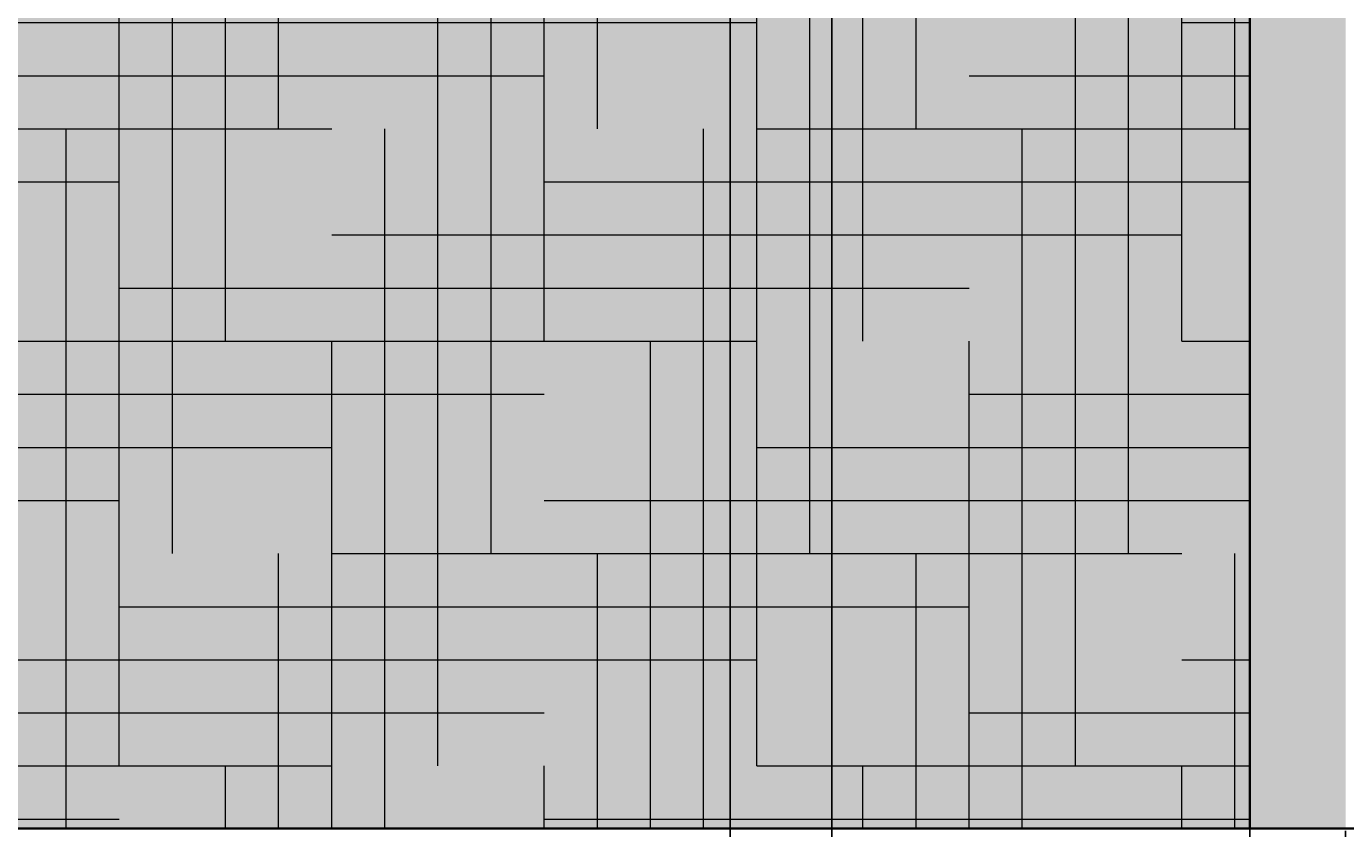
# Model space of a CAD drawing. Units: feet. Extents: x 2695 to 2912, y 795 to 1139.
# Tile 4 of 83: x 2734 to 2774, y 811 to 835. Entities that reach past the tile are written whole.
import ezdxf

# ---------------------------------------------------------------- set-up
doc = ezdxf.new("R2010")
doc.units = ezdxf.units.FT
for name, color, linetype, lineweight in [('A-ANNO-DIMS', 2, 'Continuous', 18), ('A-ELEV', 7, 'Continuous', 35), ('A-ELEV-PATT', 252, 'Continuous', 13)]:
    doc.layers.add(name, color=color, linetype=linetype, lineweight=lineweight)
doc.styles.get("Standard").update_dxf_attribs({"font": 'arial.ttf'})
doc.dimstyles.get("Standard").update_dxf_attribs({"dimtxt": 0.18, "dimasz": 0.18, "dimexe": 0.18, "dimexo": 0.0625, "dimgap": 0.09, "dimtad": 0, "dimtih": 1, "dimtoh": 1, "dimdec": 1, "dimzin": 0, "dimdsep": 46, "dimlunit": 3, "dimtxsty": 'Standard', "dimcen": 0.09, "dimadec": 0, "dimazin": 0, "dimtfac": 1, "dimtdec": 1, "dimtofl": 0, "dimtmove": 0, "dimatfit": 3, "dimfxl": 1, "dimtolj": 1, "dimtzin": 0, "dimarcsym": 0})

# ---------------------------------------------------------------- blocks, each defined once
blk = doc.blocks.new('*D3')
at = {"layer": 'A-ANNO-DIMS', "color": 0, "lineweight": -2, "transparency": 16777216}
for p, q in [((2724.189, 874.795), (2724.189, 794.976)), ((2758.151, 874.795), (2758.151, 794.976)), ((2724.369, 795.156), (2740.777, 795.156)), ((2757.971, 795.156), (2741.564, 795.156))]:
    blk.add_line(p, q, dxfattribs=at)
at = {"layer": 'A-ANNO-DIMS', "color": 0, "transparency": 16777216}
for points in [[(2724.369, 795.186), (2724.369, 795.126), (2724.189, 795.156)], [(2757.971, 795.186), (2757.971, 795.126), (2758.151, 795.156)]]:
    blk.add_solid(points, dxfattribs=at)
at = {"layer": 'Defpoints', "color": 0, "transparency": 16777216}
for p in [(2724.189, 874.857), (2758.151, 874.857), (2758.151, 795.156)]:
    blk.add_point(p, dxfattribs=at)
at = {"layer": 'A-ANNO-DIMS', "color": 0, "transparency": 16777216, "insert": (2741.17, 795.156), "char_height": 0.18, "attachment_point": 5}
blk.add_mtext('\\A1;33.96', dxfattribs=at)
blk = doc.blocks.new('*D4')
at = {"layer": 'A-ANNO-DIMS', "color": 0, "lineweight": -2, "transparency": 16777216}
for p, q in [((2758.151, 874.795), (2758.151, 794.976)), ((2773.503, 810.868), (2773.503, 794.976)), ((2758.331, 795.156), (2765.441, 795.156)), ((2773.323, 795.156), (2766.213, 795.156))]:
    blk.add_line(p, q, dxfattribs=at)
at = {"layer": 'A-ANNO-DIMS', "color": 0, "transparency": 16777216}
for points in [[(2758.331, 795.186), (2758.331, 795.126), (2758.151, 795.156)], [(2773.323, 795.186), (2773.323, 795.126), (2773.503, 795.156)]]:
    blk.add_solid(points, dxfattribs=at)
at = {"layer": 'Defpoints', "color": 0, "transparency": 16777216}
for p in [(2758.151, 874.857), (2773.503, 810.931), (2773.503, 795.156)]:
    blk.add_point(p, dxfattribs=at)
at = {"layer": 'A-ANNO-DIMS', "color": 0, "transparency": 16777216, "insert": (2765.827, 795.156), "char_height": 0.18, "attachment_point": 5}
blk.add_mtext('\\A1;15.35', dxfattribs=at)
blk = doc.blocks.new('*D13')
at = {"layer": 'A-ANNO-DIMS', "color": 0, "lineweight": -2, "transparency": 16777216}
for p, q in [((2758.214, 874.857), (2911.424, 874.857)), ((2911.244, 874.677), (2911.244, 843.076)), ((2911.244, 811.111), (2911.244, 842.712)), ((2890.699, 810.931), (2911.424, 810.931))]:
    blk.add_line(p, q, dxfattribs=at)
at = {"layer": 'A-ANNO-DIMS', "color": 0, "transparency": 16777216}
for points in [[(2911.214, 874.677), (2911.274, 874.677), (2911.244, 874.857)], [(2911.214, 811.111), (2911.274, 811.111), (2911.244, 810.931)]]:
    blk.add_solid(points, dxfattribs=at)
at = {"layer": 'Defpoints', "color": 0, "transparency": 16777216}
for p in [(2758.151, 874.857), (2911.244, 874.857), (2890.636, 810.931)]:
    blk.add_point(p, dxfattribs=at)
at = {"layer": 'A-ANNO-DIMS', "color": 0, "transparency": 16777216, "insert": (2911.244, 842.894), "char_height": 0.18, "attachment_point": 5}
blk.add_mtext('\\A1;63.93', dxfattribs=at)
blk = doc.blocks.new('*D24')
at = {"layer": 'A-ANNO-DIMS', "color": 0, "lineweight": -2, "transparency": 16777216}
for p, q in [((2730.708, 936.868), (2730.708, 794.976)), ((2755.112, 936.868), (2755.112, 794.976)), ((2730.888, 795.156), (2742.446, 795.156)), ((2754.932, 795.156), (2743.375, 795.156))]:
    blk.add_line(p, q, dxfattribs=at)
at = {"layer": 'A-ANNO-DIMS', "color": 0, "transparency": 16777216}
for points in [[(2730.888, 795.186), (2730.888, 795.126), (2730.708, 795.156)], [(2754.932, 795.186), (2754.932, 795.126), (2755.112, 795.156)]]:
    blk.add_solid(points, dxfattribs=at)
at = {"layer": 'Defpoints', "color": 0, "transparency": 16777216}
for p in [(2730.708, 936.931), (2755.112, 936.931), (2755.112, 795.156)]:
    blk.add_point(p, dxfattribs=at)
at = {"layer": 'A-ANNO-DIMS', "color": 0, "transparency": 16777216, "insert": (2742.91, 795.156), "char_height": 0.18, "attachment_point": 5}
blk.add_mtext('\\A1;24.404', dxfattribs=at)
blk = doc.blocks.new('*D25')
at = {"layer": 'A-ANNO-DIMS', "color": 0, "lineweight": -2, "transparency": 16777216}
for p, q in [((2755.112, 936.868), (2755.112, 794.976)), ((2770.636, 936.868), (2770.636, 794.976)), ((2755.292, 795.156), (2762.419, 795.156)), ((2770.456, 795.156), (2763.329, 795.156))]:
    blk.add_line(p, q, dxfattribs=at)
at = {"layer": 'A-ANNO-DIMS', "color": 0, "transparency": 16777216}
for points in [[(2755.292, 795.186), (2755.292, 795.126), (2755.112, 795.156)], [(2770.456, 795.186), (2770.456, 795.126), (2770.636, 795.156)]]:
    blk.add_solid(points, dxfattribs=at)
at = {"layer": 'Defpoints', "color": 0, "transparency": 16777216}
for p in [(2755.112, 936.931), (2770.636, 936.931), (2770.636, 795.156)]:
    blk.add_point(p, dxfattribs=at)
at = {"layer": 'A-ANNO-DIMS', "color": 0, "transparency": 16777216, "insert": (2762.874, 795.156), "char_height": 0.18, "attachment_point": 5}
blk.add_mtext('\\A1;15.524', dxfattribs=at)

msp = doc.modelspace()

# ---------------------------------------------------------------- hatches: boundary and pattern name
at = {"layer": 'A-ELEV-PATT'}
h = msp.add_hatch(color=256, dxfattribs=at)
h.set_gradient(color1=(147, 149, 152), color2=(147, 149, 152), tint=1)
h.paths.add_polyline_path([(2770.6361, 1118.4096), (2710.6361, 1118.4096), (2710.6361, 1062.9306), (2770.6361, 1062.9306)])
h.paths.add_polyline_path([(2890.6361, 1103.3378), (2770.6361, 1103.3378), (2770.6361, 1062.9306), (2890.6361, 1062.9306)])
h.paths.add_polyline_path([(2730.7081, 1048.1052), (2755.1125, 1048.1052), (2755.1125, 936.9306), (2770.6361, 936.9306), (2770.6361, 1050.3105), (2715.8852, 1050.3105), (2715.8852, 936.9306), (2730.7081, 936.9306)])
h.paths.add_polyline_path([(2890.6361, 1050.3105), (2770.6361, 1050.3105), (2770.6361, 971.9673), (2778.0341, 971.9673), (2778.0341, 1020.8235), (2843.575, 1020.8235), (2843.575, 971.9673), (2890.6361, 971.9673)])
h.paths.add_polyline_path([(2888.1882, 970.7156), (2843.575, 970.7156), (2843.575, 964.8267), (2888.1882, 964.8267)])
h.paths.add_polyline_path([(2888.1882, 964.1328), (2843.575, 964.1328), (2843.575, 956.614), (2888.1882, 956.614)])
h.paths.add_polyline_path([(2888.1882, 955.9202), (2843.575, 955.9202), (2843.575, 949.2892), (2888.1882, 949.2892)])
h.paths.add_polyline_path([(2888.1882, 948.5954), (2843.575, 948.5954), (2843.575, 941.3507), (2888.1882, 941.3507)])
h.paths.add_polyline_path([(2888.1882, 940.6569), (2843.575, 940.6569), (2843.575, 936.9306), (2888.1882, 936.9306)])
h.paths.add_polyline_path([(2890.6361, 970.7156), (2888.9368, 970.7156), (2888.9368, 964.8267), (2890.6361, 964.8267)])
h.paths.add_polyline_path([(2890.6361, 964.1328), (2888.9368, 964.1328), (2888.9368, 956.614), (2890.6361, 956.614)])
h.paths.add_polyline_path([(2890.6361, 955.9202), (2888.9368, 955.9202), (2888.9368, 949.2892), (2890.6361, 949.2892)])
h.paths.add_polyline_path([(2890.6361, 940.6569), (2888.9368, 940.6569), (2888.9368, 936.9306), (2890.6361, 936.9306)])
h.paths.add_polyline_path([(2890.6361, 948.5954), (2888.9368, 948.5954), (2888.9368, 941.3507), (2890.6361, 941.3507)])
h.paths.add_polyline_path([(2772.5216, 970.7156), (2770.6361, 970.7156), (2770.6361, 964.8267), (2772.5216, 964.8267)])
h.paths.add_polyline_path([(2772.5216, 964.1328), (2770.6361, 964.1328), (2770.6361, 956.614), (2772.5216, 956.614)])
h.paths.add_polyline_path([(2772.5216, 955.9202), (2770.6361, 955.9202), (2770.6361, 949.2892), (2772.5216, 949.2892)])
h.paths.add_polyline_path([(2772.5216, 948.5954), (2770.6361, 948.5954), (2770.6361, 941.3507), (2772.5216, 941.3507)])
h.paths.add_polyline_path([(2772.5216, 940.6569), (2770.6361, 940.6569), (2770.6361, 936.9306), (2772.5216, 936.9306)])
h.paths.add_polyline_path([(2778.0341, 940.6569), (2773.2702, 940.6569), (2773.2702, 936.9306), (2778.0341, 936.9306)])
h.paths.add_polyline_path([(2778.0341, 970.7156), (2773.2702, 970.7156), (2773.2702, 964.8267), (2778.0341, 964.8267)])
h.paths.add_polyline_path([(2778.0341, 964.1328), (2773.2702, 964.1328), (2773.2702, 956.614), (2778.0341, 956.614)])
h.paths.add_polyline_path([(2778.0341, 955.9202), (2773.2702, 955.9202), (2773.2702, 949.2892), (2778.0341, 949.2892)])
h.paths.add_polyline_path([(2778.0341, 948.5954), (2773.2702, 948.5954), (2773.2702, 941.3507), (2778.0341, 941.3507)])
h.paths.add_polyline_path([(2810.0407, 940.6569), (2780.0341, 940.6569), (2780.0341, 936.9306), (2810.0407, 936.9306)])
h.paths.add_polyline_path([(2890.6361, 924.3105), (2770.6361, 924.3105), (2770.6361, 810.9306), (2773.5029, 810.9306), (2773.5029, 905.5143), (2805.9398, 905.5143), (2838.3767, 905.5143), (2838.3767, 810.9306), (2890.6361, 810.9306)])
h = msp.add_hatch(color=256, dxfattribs=at)
h.set_gradient(color1=(255, 255, 255))
h.paths.add_polyline_path([(2770.6361, 924.3105), (2716.5358, 924.3105), (2716.5358, 810.9306), (2770.6361, 810.9306)])
h.paths.add_polyline_path([(2758.1515, 902.577), (2758.1515, 874.8571), (2724.1893, 874.8571), (2724.1893, 902.577)], flags=16)
h.paths.add_polyline_path([(2756.1515, 900.577), (2756.1515, 876.8571), (2726.1893, 876.8571), (2726.1893, 900.577)], flags=0)
h.paths.add_polyline_path([(2740.7302, 900.577), (2741.6105, 900.577), (2741.6105, 876.8571), (2740.7302, 876.8571)], flags=0)
h = msp.add_hatch(dxfattribs=at)
h.set_pattern_fill('HOUND', color=256, style=0)
h.paths.add_polyline_path([(2770.6361, 924.3105), (2716.5358, 924.3105), (2716.5358, 810.9306), (2770.6361, 810.9306)])
h.paths.add_polyline_path([(2724.1893, 874.8571), (2724.1893, 902.577), (2758.1515, 902.577), (2758.1515, 874.8571)], flags=16)
h.paths.add_polyline_path([(2756.1515, 876.8571), (2726.1893, 876.8571), (2726.1893, 900.577), (2756.1515, 900.577)], flags=0)
h.paths.add_polyline_path([(2741.6105, 876.8571), (2740.7302, 876.8571), (2740.7302, 900.577), (2741.6105, 900.577)], flags=0)

# ---------------------------------------------------------------- linework, layer by layer
at = {"layer": 'A-ELEV'}
for p, q in [((2770.6361, 924.3105), (2770.6361, 810.9306)), ((2770.6361, 810.9306), (2770.6361, 924.3105)), ((2710.6361, 810.9306), (2890.6361, 810.9306)), ((2710.6361, 810.9306), (2890.6361, 810.9306)), ((2710.6361, 810.9306), (2895.4426, 810.9306)), ((2716.5358, 810.9306), (2770.6361, 810.9306))]:
    msp.add_line(p, q, dxfattribs=at)
msp.add_lwpolyline([(2716.5358, 924.3105), (2770.6361, 924.3105), (2770.6361, 810.9306), (2716.5358, 810.9306)], close=True, dxfattribs=at)

# ---------------------------------------------------------------- dimensions: what is measured, and where the dimension line sits
at = {"layer": 'A-ANNO-DIMS'}
for base, p1, p2, override, picture, middle in [((2755.1125, 795.1556), (2730.7081, 936.9306), (2755.1125, 936.9306), {"dimdec": 3, "dimlfac": 1, "dimrnd": 0, "dimzin": 0, "dimdsep": 46, "dimlunit": 2}, '*D24', (2742.9103, 795.1556)), ((2770.6361, 795.1556), (2755.1125, 936.9306), (2770.6361, 936.9306), {"dimdec": 3, "dimlfac": 1, "dimrnd": 0, "dimzin": 0, "dimdsep": 46, "dimlunit": 2}, '*D25', (2762.8743, 795.1556)), ((2758.1515, 795.1556), (2724.1893, 874.8571), (2758.1515, 874.8571), {"dimdec": 2, "dimlfac": 1, "dimrnd": 0, "dimzin": 0, "dimdsep": 46, "dimlunit": 2}, '*D3', (2741.1704, 795.1556)), ((2773.5029, 795.1556), (2758.1515, 874.8571), (2773.5029, 810.9306), {"dimdec": 2, "dimlfac": 1, "dimrnd": 0, "dimzin": 0, "dimdsep": 46, "dimlunit": 2}, '*D4', (2765.8272, 795.1556))]:
    dim = msp.add_linear_dim(base=base, p1=p1, p2=p2, dimstyle='Standard', override=override, dxfattribs=at)
    dim.commit()
    dim.dimension.update_dxf_attribs({"geometry": picture, "text_midpoint": middle})
dim = msp.add_linear_dim(base=(2911.2444, 874.8571), p1=(2890.6361, 810.9306), p2=(2758.1515, 874.8571), angle=90, dimstyle='Standard', override={"dimdec": 2, "dimlfac": 1, "dimrnd": 0, "dimzin": 0, "dimdsep": 46, "dimlunit": 2}, dxfattribs=at)
dim.commit()
dim.dimension.update_dxf_attribs({"geometry": '*D13', "text_midpoint": (2911.2444, 842.8938)})

doc.saveas('drawing.dxf')
